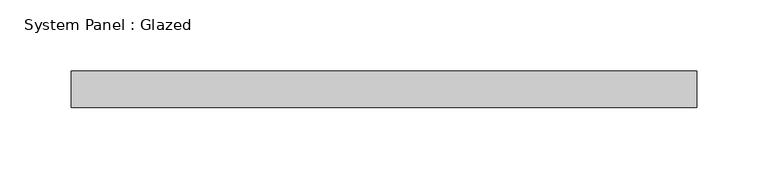
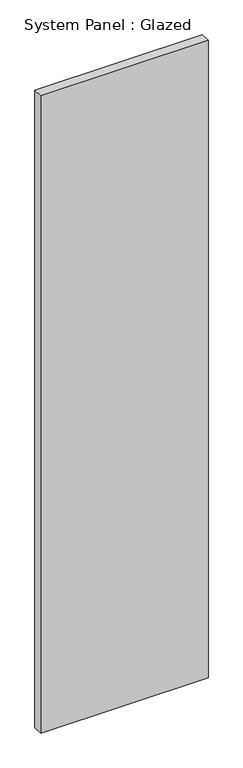
"""IFC4 building model written with IfcOpenShell, lengths in millimetres: plate geometry, System Panel : Glazed."""

from ifc_helpers import new_model, si_unit, origin, origin_with_axes, place, context, project, spatial, polyline, outline, extrude, source, transform, mapped, element, save


def system_panel_glazed_0e598201(model_context):
    return source(origin(), model_context, "Body", "SweptSolid", [
        extrude(outline(polyline([(219.075, 19.05), (-219.075, 19.05), (-219.075, 44.45), (219.075, 44.45), (219.075, 19.05)])), origin_with_axes(), (0.0, 0.0, 1.0), 1762.1776273),
    ])


if __name__ == "__main__":
    model = new_model("IFC4")
    model_context = context("Model", 3, world=origin())
    ifc_project = project(units=[si_unit("LENGTHUNIT", "METRE", prefix="MILLI")], contexts=[model_context])
    site = spatial("IfcSite", under=ifc_project)
    building = spatial("IfcBuilding", under=site)
    placement = place(None, origin())
    system_panel_glazed_shape = system_panel_glazed_0e598201(model_context)
    element("IfcPlate", 1, ObjectType="System Panel : Glazed", at=placement, inside=building, context=model_context, shape_type="MappedRepresentation", body=[
        mapped(system_panel_glazed_shape, transform((0.0, 0.0, 0.0), x_axis=(1.0, 0.0, 0.0), y_axis=(0.0, 1.0, 0.0), z_axis=(0.0, 0.0, 1.0))),
    ])
    save(model, "model.ifc")

# Revit data of these elements
# Type "System Panel : Glazed"
#   Construction Type Id = "GSP4R"
#   Analytic Construction = "1/8 in Pilkington single glazing"
#   Visual Light Transmittance = 0.9
#   Solar Heat Gain Coefficient = 0.86
#   Heat Transfer Coefficient (U) = 1.18115 BTU/(h·ft²·°F)
#   Define Thermal Properties by = 1
# Element 1 (IfcPlate, "System Panel : Glazed")
#   Materials on its faces: "Glass"
# Materials
#   "Glass": class "Glass", colour RGB 0 128 192, transparency 0.75, Description = "Soda Lime Glass", Cost = 0
